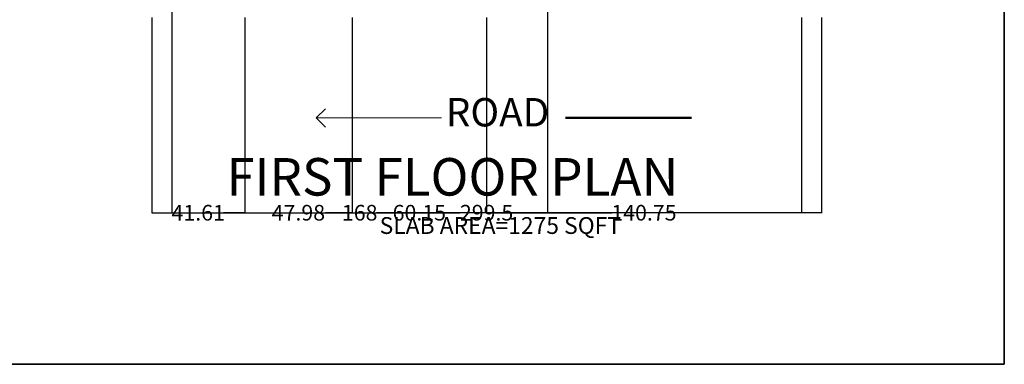
# Model space of a CAD drawing. Units: inches. Extents: x 1381 to 2246, y 1317 to 2168.
# Tile 9 of 15: x 1804 to 2244, y 1317 to 1471. Entities that reach past the tile are written whole.
import ezdxf

# ---------------------------------------------------------------- set-up
doc = ezdxf.new("R2010")
doc.units = ezdxf.units.IN
doc.header["$MEASUREMENT"] = 0
doc.layers.get('0').update_dxf_attribs({"color": 253})
for name, color, linetype, lineweight in [('A-ANNO-DIMS', 2, 'Continuous', 18), ('A-ANNO-SYMB', 7, 'Continuous', 18), ('A-ANNO-TEXT', 7, 'Continuous', 18), ('A-ANNO-TTLB', 7, 'Continuous', 35), ('A-AREA-IDEN', 3, 'Continuous', 25), ('A-WALL', 7, 'Continuous', 50)]:
    doc.layers.add(name, color=color, linetype=linetype, lineweight=lineweight)
doc.styles.get("Standard").update_dxf_attribs({"font": 'arial.ttf'})
doc.dimstyles.get("Standard").update_dxf_attribs({"dimtxt": 7, "dimasz": 0.18, "dimexe": 0.18, "dimexo": 0.0625, "dimgap": 0.09, "dimtad": 0, "dimtih": 1, "dimtoh": 1, "dimdec": 1, "dimzin": 0, "dimdsep": 46, "dimlunit": 3, "dimtxsty": 'Standard', "dimcen": 0.09, "dimadec": 0, "dimazin": 0, "dimtfac": 1, "dimtdec": 1, "dimtofl": 0, "dimtmove": 0, "dimatfit": 3, "dimfxl": 1, "dimtolj": 1, "dimtzin": 0, "dimarcsym": 0})

# ---------------------------------------------------------------- blocks, each defined once
blk = doc.blocks.new('ARROW-ROAD')
for q in [(4.11, 8.25), (56.05, 4.15), (4.15, 0)]:
    blk.add_line((0, 4.15), q)
blk = doc.blocks.new('*D75')
at = {"layer": 'A-ANNO-DIMS', "color": 0, "lineweight": -2, "transparency": 16777216}
for p, q in [((1862.81, 1471.85), (1862.81, 1384.36)), ((2162.31, 1471.85), (2162.31, 1384.36)), ((1862.99, 1384.54), (2000.57, 1384.54)), ((2162.13, 1384.54), (2024.54, 1384.54))]:
    blk.add_line(p, q, dxfattribs=at)
at = {"layer": 'A-ANNO-DIMS', "color": 0, "transparency": 16777216}
for points in [[(1862.99, 1384.57), (1862.99, 1384.51), (1862.81, 1384.54)], [(2162.13, 1384.57), (2162.13, 1384.51), (2162.31, 1384.54)]]:
    blk.add_solid(points, dxfattribs=at)
at = {"layer": 'Defpoints', "color": 0, "transparency": 16777216}
for p in [(1862.81, 1471.92), (2162.31, 1471.92), (2162.31, 1384.54)]:
    blk.add_point(p, dxfattribs=at)
at = {"layer": 'A-ANNO-DIMS', "color": 0, "transparency": 16777216, "insert": (2012.56, 1384.54), "char_height": 7, "attachment_point": 5}
blk.add_mtext('\\A1;299.5', dxfattribs=at)
blk = doc.blocks.new('*D88')
at = {"layer": 'A-ANNO-DIMS', "color": 0, "lineweight": -2, "transparency": 16777216}
for p, q in [((1862.81, 1471.85), (1862.81, 1384.36)), ((1904.42, 1471.85), (1904.42, 1384.36)), ((1862.99, 1384.54), (1872.25, 1384.54)), ((1904.24, 1384.54), (1894.98, 1384.54))]:
    blk.add_line(p, q, dxfattribs=at)
at = {"layer": 'A-ANNO-DIMS', "color": 0, "transparency": 16777216}
for points in [[(1862.99, 1384.57), (1862.99, 1384.51), (1862.81, 1384.54)], [(1904.24, 1384.57), (1904.24, 1384.51), (1904.42, 1384.54)]]:
    blk.add_solid(points, dxfattribs=at)
at = {"layer": 'Defpoints', "color": 0, "transparency": 16777216}
for p in [(1862.81, 1471.92), (1904.42, 1471.92), (1904.42, 1384.54)]:
    blk.add_point(p, dxfattribs=at)
at = {"layer": 'A-ANNO-DIMS', "color": 0, "transparency": 16777216, "insert": (1883.61, 1384.54), "char_height": 7, "attachment_point": 5}
blk.add_mtext('\\A1;41.61', dxfattribs=at)
blk = doc.blocks.new('*D89')
at = {"layer": 'A-ANNO-DIMS', "color": 0, "lineweight": -2, "transparency": 16777216}
for p, q in [((1904.42, 1471.85), (1904.42, 1384.36)), ((1952.4, 1471.85), (1952.4, 1384.36)), ((1904.6, 1384.54), (1916.36, 1384.54)), ((1952.22, 1384.54), (1940.46, 1384.54))]:
    blk.add_line(p, q, dxfattribs=at)
at = {"layer": 'A-ANNO-DIMS', "color": 0, "transparency": 16777216}
for points in [[(1904.6, 1384.57), (1904.6, 1384.51), (1904.42, 1384.54)], [(1952.22, 1384.57), (1952.22, 1384.51), (1952.4, 1384.54)]]:
    blk.add_solid(points, dxfattribs=at)
at = {"layer": 'Defpoints', "color": 0, "transparency": 16777216}
for p in [(1904.42, 1471.92), (1952.4, 1471.92), (1952.4, 1384.54)]:
    blk.add_point(p, dxfattribs=at)
at = {"layer": 'A-ANNO-DIMS', "color": 0, "transparency": 16777216, "insert": (1928.41, 1384.54), "char_height": 7, "attachment_point": 5}
blk.add_mtext('\\A1;47.98', dxfattribs=at)
blk = doc.blocks.new('*D90')
at = {"layer": 'A-ANNO-DIMS', "color": 0, "lineweight": -2, "transparency": 16777216}
for p, q in [((1952.4, 1471.85), (1952.4, 1384.36)), ((2012.56, 1471.85), (2012.56, 1384.36)), ((1952.58, 1384.54), (1970.53, 1384.54)), ((2012.38, 1384.54), (1994.42, 1384.54))]:
    blk.add_line(p, q, dxfattribs=at)
at = {"layer": 'A-ANNO-DIMS', "color": 0, "transparency": 16777216}
for points in [[(1952.58, 1384.57), (1952.58, 1384.51), (1952.4, 1384.54)], [(2012.38, 1384.57), (2012.38, 1384.51), (2012.56, 1384.54)]]:
    blk.add_solid(points, dxfattribs=at)
at = {"layer": 'Defpoints', "color": 0, "transparency": 16777216}
for p in [(1952.4, 1471.92), (2012.56, 1471.92), (2012.56, 1384.54)]:
    blk.add_point(p, dxfattribs=at)
at = {"layer": 'A-ANNO-DIMS', "color": 0, "transparency": 16777216, "insert": (1982.48, 1384.54), "char_height": 7, "attachment_point": 5}
blk.add_mtext('\\A1;60.15', dxfattribs=at)
blk = doc.blocks.new('*D91')
at = {"layer": 'A-ANNO-DIMS', "color": 0, "lineweight": -2, "transparency": 16777216}
for p, q in [((2012.56, 1471.85), (2012.56, 1384.36)), ((2153.31, 1471.85), (2153.31, 1384.36)), ((2012.74, 1384.54), (2068.61, 1384.54)), ((2153.13, 1384.54), (2097.25, 1384.54))]:
    blk.add_line(p, q, dxfattribs=at)
at = {"layer": 'A-ANNO-DIMS', "color": 0, "transparency": 16777216}
for points in [[(2012.74, 1384.57), (2012.74, 1384.51), (2012.56, 1384.54)], [(2153.13, 1384.57), (2153.13, 1384.51), (2153.31, 1384.54)]]:
    blk.add_solid(points, dxfattribs=at)
at = {"layer": 'Defpoints', "color": 0, "transparency": 16777216}
for p in [(2012.56, 1471.92), (2153.31, 1471.92), (2153.31, 1384.54)]:
    blk.add_point(p, dxfattribs=at)
at = {"layer": 'A-ANNO-DIMS', "color": 0, "transparency": 16777216, "insert": (2082.93, 1384.54), "char_height": 7, "attachment_point": 5}
blk.add_mtext('\\A1;140.75', dxfattribs=at)
blk = doc.blocks.new('*D92')
at = {"layer": 'A-ANNO-DIMS', "color": 0, "lineweight": -2, "transparency": 16777216}
for p, q in [((1871.81, 1578.35), (1871.81, 1384.36)), ((2039.81, 1578.35), (2039.81, 1384.36)), ((1871.99, 1384.54), (1948.3, 1384.54)), ((2039.63, 1384.54), (1963.31, 1384.54))]:
    blk.add_line(p, q, dxfattribs=at)
at = {"layer": 'A-ANNO-DIMS', "color": 0, "transparency": 16777216}
for points in [[(1871.99, 1384.57), (1871.99, 1384.51), (1871.81, 1384.54)], [(2039.63, 1384.57), (2039.63, 1384.51), (2039.81, 1384.54)]]:
    blk.add_solid(points, dxfattribs=at)
at = {"layer": 'Defpoints', "color": 0, "transparency": 16777216}
for p in [(1871.81, 1578.42), (2039.81, 1578.42), (2039.81, 1384.54)]:
    blk.add_point(p, dxfattribs=at)
at = {"layer": 'A-ANNO-DIMS', "color": 0, "transparency": 16777216, "insert": (1955.81, 1384.54), "char_height": 7, "attachment_point": 5}
blk.add_mtext('\\A1;168', dxfattribs=at)

msp = doc.modelspace()

# ---------------------------------------------------------------- linework, layer by layer
at = {"layer": 'A-ANNO-TTLB'}
for p, q in [((2244.072, 2167.8236), (2244.072, 1316.7761)), ((2244.072, 1316.7761), (1380.9518, 1316.7761))]:
    msp.add_line(p, q, dxfattribs=at)
at = {"layer": 'A-WALL'}
msp.add_line((2047.8971, 1426.938), (2104.1953, 1426.938), dxfattribs=at)

# ---------------------------------------------------------------- block references
at = {"layer": 'A-ANNO-SYMB'}
msp.add_blockref('ARROW-ROAD', (1936.3993, 1422.791), dxfattribs=at)

# ---------------------------------------------------------------- texts
at = {"layer": 'A-ANNO-TEXT'}
for s, height, p in [('ROAD', 12.68973, (1994.3405, 1423.1241)), ('SLAB AREA=1275 SQFT', 7.495394, (1964.736, 1375.0646))]:
    msp.add_text(s, height=height, dxfattribs=at).set_placement(p)
at = {"layer": 'A-AREA-IDEN'}
msp.add_text('FIRST FLOOR PLAN', height=16.755681, dxfattribs=at).set_placement((1896.1981, 1392.2038))

# ---------------------------------------------------------------- dimensions: what is measured, and where the dimension line sits
at = {"layer": 'A-ANNO-DIMS'}
for base, p1, p2, override, picture, middle in [((2039.8052, 1384.5407), (1871.8052, 1578.4163), (2039.8052, 1578.4163), {"dimdec": 0, "dimlfac": 1, "dimrnd": 0, "dimzin": 0, "dimdsep": 46, "dimlunit": 2}, '*D92', (1955.8052, 1384.5407)), ((2162.3052, 1384.5407), (1862.8052, 1471.9163), (2162.3052, 1471.9163), {"dimdec": 1, "dimlfac": 1, "dimrnd": 0, "dimzin": 0, "dimdsep": 46, "dimlunit": 2}, '*D75', (2012.5552, 1384.5407)), ((1904.4174, 1384.5407), (1862.8052, 1471.9163), (1904.4174, 1471.9163), {"dimdec": 2, "dimlfac": 1, "dimrnd": 0, "dimzin": 0, "dimdsep": 46, "dimlunit": 2}, '*D88', (1883.6113, 1384.5407)), ((1952.401, 1384.5407), (1904.4174, 1471.9163), (1952.401, 1471.9163), {"dimdec": 2, "dimlfac": 1, "dimrnd": 0, "dimzin": 0, "dimdsep": 46, "dimlunit": 2}, '*D89', (1928.4092, 1384.5407)), ((2012.5552, 1384.5407), (1952.401, 1471.9163), (2012.5552, 1471.9163), {"dimdec": 2, "dimlfac": 1, "dimrnd": 0, "dimzin": 0, "dimdsep": 46, "dimlunit": 2}, '*D90', (1982.4781, 1384.5407)), ((2153.3052, 1384.5407), (2012.5552, 1471.9163), (2153.3052, 1471.9163), {"dimdec": 2, "dimlfac": 1, "dimrnd": 0, "dimzin": 0, "dimdsep": 46, "dimlunit": 2}, '*D91', (2082.9302, 1384.5407))]:
    dim = msp.add_linear_dim(base=base, p1=p1, p2=p2, dimstyle='Standard', override=override, dxfattribs=at)
    dim.commit()
    dim.dimension.update_dxf_attribs({"geometry": picture, "text_midpoint": middle})

doc.saveas('drawing.dxf')
